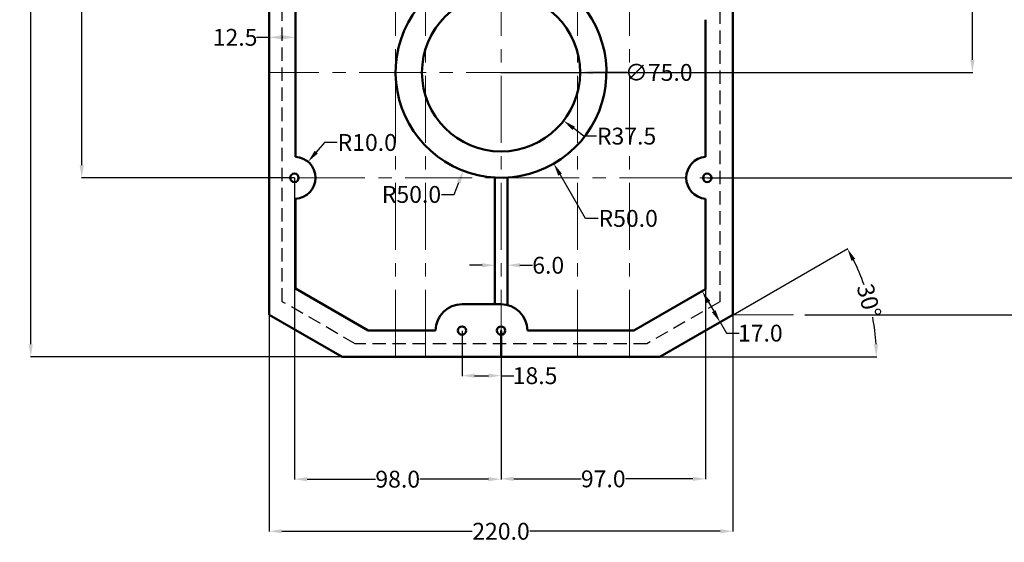
# Model space of a CAD drawing. Units: inches. Extents: x 11765 to 12471, y 10149 to 10793.
# Tile 1 of 8: x 11765 to 12232, y 10149 to 10397. Entities that reach past the tile are written whole.
import ezdxf

# ---------------------------------------------------------------- set-up
doc = ezdxf.new("R2010")
doc.units = ezdxf.units.IN
doc.header["$MEASUREMENT"] = 0
doc.linetypes.add('CENTER', pattern=[50.8, 31.75, -6.35, 6.35, -6.35])
doc.linetypes.add('HIDDEN', pattern=[9.525, 6.35, -3.175])
for name, color, linetype, lineweight in [('M-CNTR', 30, 'CENTER', 18), ('M-DIMS', 2, 'Continuous', 25), ('M-HIDN', 41, 'HIDDEN', 25), ('M-OUTL', 7, 'Continuous', 50)]:
    doc.layers.add(name, color=color, linetype=linetype, lineweight=lineweight)
doc.styles.get("Standard").update_dxf_attribs({"font": 'arial.ttf'})
doc.dimstyles.get("Standard").update_dxf_attribs({"dimtxt": 8, "dimasz": 6, "dimexe": 0.18, "dimexo": 0.0625, "dimgap": 0.09, "dimtad": 0, "dimtoh": 1, "dimdec": 1, "dimzin": 0, "dimdsep": 46, "dimtxsty": 'Standard', "dimcen": 0.09, "dimadec": 0, "dimazin": 0, "dimtfac": 1, "dimtdec": 1, "dimtofl": 0, "dimtmove": 0, "dimatfit": 3, "dimfxl": 1, "dimtolj": 1, "dimtzin": 0, "dimarcsym": 0})

# ---------------------------------------------------------------- blocks, each defined once
blk = doc.blocks.new('*D6')
at = {"layer": 'Defpoints', "color": 0, "transparency": 16777216}
for p in [(11882.91, 10712.15), (11769.87, 10237.15), (11917.55, 10237.15)]:
    blk.add_point(p, dxfattribs=at)
at = {"layer": 'M-DIMS', "color": 0, "lineweight": -2, "transparency": 16777216}
for p, q in [((11882.85, 10712.15), (11769.69, 10712.15)), ((11769.87, 10706.15), (11769.87, 10488.38)), ((11769.87, 10243.15), (11769.87, 10460.91)), ((11917.49, 10237.15), (11769.69, 10237.15))]:
    blk.add_line(p, q, dxfattribs=at)
at = {"layer": 'M-DIMS', "color": 0, "transparency": 16777216}
for points in [[(11768.87, 10706.15), (11770.87, 10706.15), (11769.87, 10712.15)], [(11768.87, 10243.15), (11770.87, 10243.15), (11769.87, 10237.15)]]:
    blk.add_solid(points, dxfattribs=at)
at = {"layer": 'M-DIMS', "color": 0, "transparency": 16777216, "insert": (11769.87, 10474.65), "char_height": 8, "attachment_point": 5, "rotation": 90}
blk.add_mtext('\\A1;475.0', dxfattribs=at)
blk = doc.blocks.new('*D14')
at = {"layer": 'Defpoints', "color": 0, "transparency": 16777216}
for p in [(12156.23, 10592.15), (12216.5, 10592.15), (11992.91, 10372.15)]:
    blk.add_point(p, dxfattribs=at)
at = {"layer": 'M-DIMS', "color": 0, "lineweight": -2, "transparency": 16777216}
for p, q in [((12156.3, 10592.15), (12216.68, 10592.15)), ((12216.5, 10586.15), (12216.5, 10495.79)), ((12216.5, 10378.15), (12216.5, 10468.5)), ((11992.97, 10372.15), (12216.68, 10372.15))]:
    blk.add_line(p, q, dxfattribs=at)
at = {"layer": 'M-DIMS', "color": 0, "transparency": 16777216}
for points in [[(12215.5, 10586.15), (12217.5, 10586.15), (12216.5, 10592.15)], [(12215.5, 10378.15), (12217.5, 10378.15), (12216.5, 10372.15)]]:
    blk.add_solid(points, dxfattribs=at)
at = {"layer": 'M-DIMS', "color": 0, "transparency": 16777216, "insert": (12216.5, 10482.15), "char_height": 8, "attachment_point": 5, "rotation": 90}
blk.add_mtext('\\A1;220.0', dxfattribs=at)
blk = doc.blocks.new('*D15')
at = {"layer": 'Defpoints', "color": 0, "transparency": 16777216}
for p in [(12198.7, 10592.15), (12090.75, 10322.15), (12241.87, 10322.15)]:
    blk.add_point(p, dxfattribs=at)
at = {"layer": 'M-DIMS', "color": 0, "lineweight": -2, "transparency": 16777216}
for p, q in [((12198.76, 10592.15), (12242.05, 10592.15)), ((12241.87, 10586.15), (12241.87, 10470.79)), ((12241.87, 10328.15), (12241.87, 10443.5)), ((12090.81, 10322.15), (12242.05, 10322.15))]:
    blk.add_line(p, q, dxfattribs=at)
at = {"layer": 'M-DIMS', "color": 0, "transparency": 16777216}
for points in [[(12240.87, 10586.15), (12242.87, 10586.15), (12241.87, 10592.15)], [(12240.87, 10328.15), (12242.87, 10328.15), (12241.87, 10322.15)]]:
    blk.add_solid(points, dxfattribs=at)
at = {"layer": 'M-DIMS', "color": 0, "transparency": 16777216, "insert": (12241.87, 10457.15), "char_height": 8, "attachment_point": 5, "rotation": 90}
blk.add_mtext('\\A1;270.0', dxfattribs=at)
blk = doc.blocks.new('*D16')
at = {"layer": 'Defpoints', "color": 0, "transparency": 16777216}
for p in [(12136.92, 10322.15), (12136.92, 10257.15), (12239.74, 10257.15)]:
    blk.add_point(p, dxfattribs=at)
at = {"layer": 'M-DIMS', "color": 0, "lineweight": -2, "transparency": 16777216}
for p, q in [((12136.98, 10322.15), (12239.92, 10322.15)), ((12239.74, 10316.15), (12239.74, 10300.13)), ((12239.74, 10263.15), (12239.74, 10279.16)), ((12136.98, 10257.15), (12239.92, 10257.15))]:
    blk.add_line(p, q, dxfattribs=at)
at = {"layer": 'M-DIMS', "color": 0, "transparency": 16777216}
for points in [[(12238.74, 10316.15), (12240.74, 10316.15), (12239.74, 10322.15)], [(12238.74, 10263.15), (12240.74, 10263.15), (12239.74, 10257.15)]]:
    blk.add_solid(points, dxfattribs=at)
at = {"layer": 'M-DIMS', "color": 0, "transparency": 16777216, "insert": (12239.74, 10289.65), "char_height": 8, "attachment_point": 5, "rotation": 90}
blk.add_mtext('\\A1;65.0', dxfattribs=at)
blk = doc.blocks.new('*D17')
at = {"layer": 'Defpoints', "color": 0, "transparency": 16777216}
for p in [(12102.91, 10257.15), (12169.38, 10254.97), (11917.55, 10237.15), (12068.27, 10237.15), (12068.27, 10237.15)]:
    blk.add_point(p, dxfattribs=at)
at = {"layer": 'M-DIMS', "color": 0, "lineweight": -2, "transparency": 16777216}
for p, q in [((12102.97, 10257.18), (12157.34, 10288.57)), ((12068.33, 10237.15), (12171.12, 10237.15))]:
    blk.add_line(p, q, dxfattribs=at)
for start, end in [(19.4324, 26.6511), (3.3489, 10.5676)]:
    blk.add_arc((12068.27, 10237.15), 102.67, start, end, dxfattribs=at)
at = {"layer": 'M-DIMS', "color": 0, "transparency": 16777216}
for points in [[(12159.15, 10282.72), (12160.91, 10283.67), (12157.18, 10288.48)], [(12171.76, 10243.17), (12169.76, 10243.11), (12170.94, 10237.15)]]:
    blk.add_solid(points, dxfattribs=at)
at = {"layer": 'M-DIMS', "color": 0, "transparency": 16777216, "insert": (12167.44, 10263.72), "char_height": 8, "attachment_point": 5, "rotation": 285}
blk.add_mtext('\\A1;30°', dxfattribs=at)
blk = doc.blocks.new('*D18')
at = {"layer": 'Defpoints', "color": 0, "transparency": 16777216}
for p in [(11882.91, 10257.15), (12102.91, 10257.15), (12102.91, 10154.4)]:
    blk.add_point(p, dxfattribs=at)
at = {"layer": 'M-DIMS', "color": 0, "lineweight": -2, "transparency": 16777216}
for p, q in [((11882.91, 10257.08), (11882.91, 10154.22)), ((12102.91, 10257.08), (12102.91, 10154.22)), ((11888.91, 10154.4), (11979.27, 10154.4)), ((12096.91, 10154.4), (12006.55, 10154.4))]:
    blk.add_line(p, q, dxfattribs=at)
at = {"layer": 'M-DIMS', "color": 0, "transparency": 16777216}
for points in [[(11888.91, 10155.4), (11888.91, 10153.4), (11882.91, 10154.4)], [(12096.91, 10155.4), (12096.91, 10153.4), (12102.91, 10154.4)]]:
    blk.add_solid(points, dxfattribs=at)
at = {"layer": 'M-DIMS', "color": 0, "transparency": 16777216, "insert": (11992.91, 10154.4), "char_height": 8, "attachment_point": 5}
blk.add_mtext('\\A1;220.0', dxfattribs=at)
blk = doc.blocks.new('*D19')
at = {"layer": 'Defpoints', "color": 0, "transparency": 16777216}
for p in [(12074.77, 10260.53), (12096.81, 10253.62), (12083.27, 10245.8)]:
    blk.add_point(p, dxfattribs=at)
at = {"layer": 'M-DIMS', "color": 0, "lineweight": -2, "transparency": 16777216}
for p, q in [((12074.82, 10260.56), (12088.46, 10268.43)), ((12091.31, 10263.15), (12093.81, 10258.82)), ((12083.32, 10245.83), (12096.96, 10253.71)), ((12096.81, 10253.62), (12099.81, 10248.42)), ((12099.81, 10248.42), (12105.81, 10248.42))]:
    blk.add_line(p, q, dxfattribs=at)
at = {"layer": 'M-DIMS', "color": 0, "transparency": 16777216}
for points in [[(12092.17, 10263.65), (12090.44, 10262.65), (12088.31, 10268.34)], [(12094.67, 10259.32), (12092.94, 10258.32), (12096.81, 10253.62)]]:
    blk.add_solid(points, dxfattribs=at)
at = {"layer": 'M-DIMS', "color": 0, "transparency": 16777216, "insert": (12115.9, 10248.42), "char_height": 8, "attachment_point": 5}
blk.add_mtext('\\A1;17.0', dxfattribs=at)
blk = doc.blocks.new('*D20')
at = {"layer": 'Defpoints', "color": 0, "transparency": 16777216}
for p in [(11894.91, 10322.15), (11992.91, 10249.65), (11992.91, 10179.12)]:
    blk.add_point(p, dxfattribs=at)
at = {"layer": 'M-DIMS', "color": 0, "lineweight": -2, "transparency": 16777216}
for p, q in [((11894.91, 10322.08), (11894.91, 10178.94)), ((11992.91, 10249.58), (11992.91, 10178.94)), ((11900.91, 10179.12), (11933.45, 10179.12)), ((11986.91, 10179.12), (11954.38, 10179.12))]:
    blk.add_line(p, q, dxfattribs=at)
at = {"layer": 'M-DIMS', "color": 0, "transparency": 16777216}
for points in [[(11900.91, 10180.12), (11900.91, 10178.12), (11894.91, 10179.12)], [(11986.91, 10180.12), (11986.91, 10178.12), (11992.91, 10179.12)]]:
    blk.add_solid(points, dxfattribs=at)
at = {"layer": 'M-DIMS', "color": 0, "transparency": 16777216, "insert": (11943.91, 10179.12), "char_height": 8, "attachment_point": 5}
blk.add_mtext('\\A1;98.0', dxfattribs=at)
blk = doc.blocks.new('*D21')
at = {"layer": 'Defpoints', "color": 0, "transparency": 16777216}
for p in [(12089.91, 10269.27), (11992.91, 10249.65), (11992.91, 10179.27)]:
    blk.add_point(p, dxfattribs=at)
at = {"layer": 'M-DIMS', "color": 0, "lineweight": -2, "transparency": 16777216}
for p, q in [((12089.91, 10269.21), (12089.91, 10179.09)), ((11992.91, 10249.58), (11992.91, 10179.09)), ((11998.91, 10179.27), (12030.95, 10179.27)), ((12083.91, 10179.27), (12051.88, 10179.27))]:
    blk.add_line(p, q, dxfattribs=at)
at = {"layer": 'M-DIMS', "color": 0, "transparency": 16777216}
for points in [[(11998.91, 10180.27), (11998.91, 10178.27), (11992.91, 10179.27)], [(12083.91, 10180.27), (12083.91, 10178.27), (12089.91, 10179.27)]]:
    blk.add_solid(points, dxfattribs=at)
at = {"layer": 'M-DIMS', "color": 0, "transparency": 16777216, "insert": (12041.41, 10179.27), "char_height": 8, "attachment_point": 5}
blk.add_mtext('\\A1;97.0', dxfattribs=at)
blk = doc.blocks.new('*D22')
at = {"layer": 'Defpoints', "color": 0, "transparency": 16777216}
for p in [(11995.91, 10280.64), (11989.91, 10277.99), (11995.91, 10277.99)]:
    blk.add_point(p, dxfattribs=at)
at = {"layer": 'M-DIMS', "color": 0, "lineweight": -2, "transparency": 16777216}
for p, q in [((11983.91, 10280.64), (11977.91, 10280.64)), ((11989.91, 10278.05), (11989.91, 10280.82)), ((11995.91, 10278.05), (11995.91, 10280.82)), ((12001.91, 10280.64), (12007.91, 10280.64))]:
    blk.add_line(p, q, dxfattribs=at)
at = {"layer": 'M-DIMS', "color": 0, "transparency": 16777216}
for points in [[(11983.91, 10281.64), (11983.91, 10279.64), (11989.91, 10280.64)], [(12001.91, 10281.64), (12001.91, 10279.64), (11995.91, 10280.64)]]:
    blk.add_solid(points, dxfattribs=at)
at = {"layer": 'M-DIMS', "color": 0, "transparency": 16777216, "insert": (12015.29, 10280.64), "char_height": 8, "attachment_point": 5}
blk.add_mtext('\\A1;6.0', dxfattribs=at)
blk = doc.blocks.new('*D23')
at = {"layer": 'Defpoints', "color": 0, "transparency": 16777216}
for p in [(11974.41, 10249.65), (11992.91, 10249.65), (11992.91, 10228.23)]:
    blk.add_point(p, dxfattribs=at)
at = {"layer": 'M-DIMS', "color": 0, "lineweight": -2, "transparency": 16777216}
for p, q in [((11974.41, 10249.58), (11974.41, 10228.05)), ((11992.91, 10249.58), (11992.91, 10228.05)), ((11980.41, 10228.23), (11986.91, 10228.23)), ((11992.91, 10228.23), (11998.91, 10228.23))]:
    blk.add_line(p, q, dxfattribs=at)
at = {"layer": 'M-DIMS', "color": 0, "transparency": 16777216}
for points in [[(11980.41, 10229.23), (11980.41, 10227.23), (11974.41, 10228.23)], [(11986.91, 10229.23), (11986.91, 10227.23), (11992.91, 10228.23)]]:
    blk.add_solid(points, dxfattribs=at)
at = {"layer": 'M-DIMS', "color": 0, "transparency": 16777216, "insert": (12009.05, 10228.23), "char_height": 8, "attachment_point": 5}
blk.add_mtext('\\A1;18.5', dxfattribs=at)
blk = doc.blocks.new('*D29')
at = {"layer": 'Defpoints', "color": 0, "transparency": 16777216}
for p in [(11794.06, 10592.15), (11889.16, 10592.15), (11894.91, 10322.15)]:
    blk.add_point(p, dxfattribs=at)
at = {"layer": 'M-DIMS', "color": 0, "lineweight": -2, "transparency": 16777216}
for p, q in [((11889.1, 10592.15), (11793.88, 10592.15)), ((11794.06, 10586.15), (11794.06, 10470.79)), ((11794.06, 10328.15), (11794.06, 10443.5)), ((11894.85, 10322.15), (11793.88, 10322.15))]:
    blk.add_line(p, q, dxfattribs=at)
at = {"layer": 'M-DIMS', "color": 0, "transparency": 16777216}
for points in [[(11793.06, 10586.15), (11795.06, 10586.15), (11794.06, 10592.15)], [(11793.06, 10328.15), (11795.06, 10328.15), (11794.06, 10322.15)]]:
    blk.add_solid(points, dxfattribs=at)
at = {"layer": 'M-DIMS', "color": 0, "transparency": 16777216, "insert": (11794.06, 10457.15), "char_height": 8, "attachment_point": 5, "rotation": 90}
blk.add_mtext('\\A1;270.0', dxfattribs=at)
blk = doc.blocks.new('*D32')
at = {"layer": 'Defpoints', "color": 0, "transparency": 16777216}
for p in [(11882.91, 10389.52), (11882.91, 10388.8), (11895.41, 10389.52)]:
    blk.add_point(p, dxfattribs=at)
at = {"layer": 'M-DIMS', "color": 0, "lineweight": -2, "transparency": 16777216}
for p, q in [((11882.91, 10388.8), (11876.91, 10388.8)), ((11882.91, 10389.45), (11882.91, 10388.62)), ((11889.41, 10388.8), (11888.91, 10388.8)), ((11895.41, 10389.45), (11895.41, 10388.62))]:
    blk.add_line(p, q, dxfattribs=at)
at = {"layer": 'M-DIMS', "color": 0, "transparency": 16777216}
for points in [[(11888.91, 10389.8), (11888.91, 10387.8), (11882.91, 10388.8)], [(11889.41, 10389.8), (11889.41, 10387.8), (11895.41, 10388.8)]]:
    blk.add_solid(points, dxfattribs=at)
at = {"layer": 'M-DIMS', "color": 0, "transparency": 16777216, "insert": (11866.78, 10388.8), "char_height": 8, "attachment_point": 5}
blk.add_mtext('\\A1;12.5', dxfattribs=at)
blk = doc.blocks.new('*D44')
at = {"layer": 'Defpoints', "color": 0, "transparency": 16777216}
for p in [(11992.91, 10372.15), (11975.02, 10325.45)]:
    blk.add_point(p, dxfattribs=at)
at = {"layer": 'M-DIMS', "color": 0, "lineweight": -2, "transparency": 16777216}
for p, q in [((11992.82, 10372.15), (11993, 10372.15)), ((11992.91, 10372.06), (11992.91, 10372.24)), ((11970.73, 10314.25), (11972.88, 10319.85)), ((11964.73, 10314.25), (11970.73, 10314.25))]:
    blk.add_line(p, q, dxfattribs=at)
at = {"layer": 'M-DIMS', "color": 0, "transparency": 16777216}
blk.add_solid([(11971.94, 10320.21), (11973.81, 10319.49), (11975.02, 10325.45)], dxfattribs=at)
at = {"layer": 'M-DIMS', "color": 0, "transparency": 16777216, "insert": (11950.44, 10314.25), "char_height": 8, "attachment_point": 5}
blk.add_mtext('\\A1;R50.0', dxfattribs=at)
blk = doc.blocks.new('*D45')
at = {"layer": 'Defpoints', "color": 0, "transparency": 16777216}
for p in [(11992.91, 10372.15), (12022.61, 10349.25)]:
    blk.add_point(p, dxfattribs=at)
at = {"layer": 'M-DIMS', "color": 0, "lineweight": -2, "transparency": 16777216}
for p, q in [((11992.82, 10372.15), (11993, 10372.15)), ((11992.91, 10372.06), (11992.91, 10372.24)), ((12032.12, 10341.93), (12027.37, 10345.59)), ((12038.12, 10341.93), (12032.12, 10341.93))]:
    blk.add_line(p, q, dxfattribs=at)
at = {"layer": 'M-DIMS', "color": 0, "transparency": 16777216}
blk.add_solid([(12027.98, 10346.38), (12026.76, 10344.8), (12022.61, 10349.25)], dxfattribs=at)
at = {"layer": 'M-DIMS', "color": 0, "transparency": 16777216, "insert": (12052.46, 10341.93), "char_height": 8, "attachment_point": 5}
blk.add_mtext('\\A1;R37.5', dxfattribs=at)
blk = doc.blocks.new('*D50')
at = {"layer": 'Defpoints', "color": 0, "transparency": 16777216}
for p in [(11901.39, 10329.76), (11894.91, 10322.15)]:
    blk.add_point(p, dxfattribs=at)
at = {"layer": 'M-DIMS', "color": 0, "lineweight": -2, "transparency": 16777216}
for p, q in [((11909.17, 10338.9), (11905.28, 10334.33)), ((11915.17, 10338.9), (11909.17, 10338.9)), ((11894.82, 10322.15), (11895, 10322.15)), ((11894.91, 10322.06), (11894.91, 10322.24))]:
    blk.add_line(p, q, dxfattribs=at)
at = {"layer": 'M-DIMS', "color": 0, "transparency": 16777216}
blk.add_solid([(11904.52, 10334.98), (11906.04, 10333.68), (11901.39, 10329.76)], dxfattribs=at)
at = {"layer": 'M-DIMS', "color": 0, "transparency": 16777216, "insert": (11929.47, 10338.9), "char_height": 8, "attachment_point": 5}
blk.add_mtext('\\A1;R10.0', dxfattribs=at)
blk = doc.blocks.new('*D67')
at = {"layer": 'Defpoints', "color": 0, "transparency": 16777216}
for p in [(11992.91, 10372.15), (12017.93, 10328.85)]:
    blk.add_point(p, dxfattribs=at)
at = {"layer": 'M-DIMS', "color": 0, "lineweight": -2, "transparency": 16777216}
for p, q in [((11992.82, 10372.15), (11993, 10372.15)), ((11992.91, 10372.06), (11992.91, 10372.24)), ((12032.94, 10302.88), (12020.93, 10323.66)), ((12038.94, 10302.88), (12032.94, 10302.88))]:
    blk.add_line(p, q, dxfattribs=at)
at = {"layer": 'M-DIMS', "color": 0, "transparency": 16777216}
blk.add_solid([(12021.79, 10324.16), (12020.06, 10323.16), (12017.93, 10328.85)], dxfattribs=at)
at = {"layer": 'M-DIMS', "color": 0, "transparency": 16777216, "insert": (12053.23, 10302.88), "char_height": 8, "attachment_point": 5}
blk.add_mtext('\\A1;R50.0', dxfattribs=at)
blk = doc.blocks.new('*D70')
at = {"layer": 'Defpoints', "color": 0, "transparency": 16777216}
for p in [(11955.41, 10372.15), (12030.41, 10372.15)]:
    blk.add_point(p, dxfattribs=at)
at = {"layer": 'M-DIMS', "color": 0, "lineweight": -2, "transparency": 16777216}
for p, q in [((11992.82, 10372.15), (11993, 10372.15)), ((11992.91, 10372.06), (11992.91, 10372.24)), ((12052.91, 10372.15), (12036.41, 10372.15))]:
    blk.add_line(p, q, dxfattribs=at)
at = {"layer": 'M-DIMS', "color": 0, "transparency": 16777216}
blk.add_solid([(12036.41, 10373.15), (12036.41, 10371.15), (12030.41, 10372.15)], dxfattribs=at)
at = {"layer": 'M-DIMS', "color": 0, "transparency": 16777216, "insert": (12067.73, 10372.15), "char_height": 8, "attachment_point": 5}
blk.add_mtext('\\A1;∅75.0', dxfattribs=at)

msp = doc.modelspace()

# ---------------------------------------------------------------- linework, layer by layer
at = {"layer": 'M-CNTR'}
for p, q in [((11942.912, 10237.146), (11942.912, 10712.146)), ((11957.122, 10237.146), (11957.122, 10712.146)), ((11992.912, 10237.146), (11992.912, 10712.146)), ((12029.232, 10237.146), (12029.232, 10712.146)), ((12053.912, 10237.146), (12053.912, 10712.146)), ((12211.379, 10372.146), (11882.912, 10372.146)), ((12182.382, 10322.146), (11882.912, 10322.146)), ((12182.382, 10257.146), (12102.912, 10257.146))]:
    msp.add_line(p, q, dxfattribs=at)
at = {"layer": 'M-HIDN'}
msp.add_lwpolyline([(12060.662, 10705.896), (12060.662, 10515.896), (12096.662, 10515.896), (12096.662, 10263.352), (12062.096, 10243.396), (11923.728, 10243.396), (11889.162, 10263.352), (11889.162, 10705.896)], close=True, dxfattribs=at)
at = {"layer": 'M-OUTL'}
for p, q in [((11882.912, 10712.146), (11882.912, 10257.146)), ((12102.912, 10257.146), (12102.912, 10522.146)), ((11895.412, 10437.158), (11895.412, 10332.133)), ((12089.912, 10332.111), (12089.912, 10397.181)), ((11989.912, 10322.146), (11989.912, 10262.146)), ((11995.912, 10322.146), (11995.912, 10262.146)), ((11895.412, 10312.158), (11895.412, 10269.559)), ((12089.912, 10269.27), (12089.912, 10312.181)), ((11895.412, 10269.559), (11929.902, 10249.646)), ((12089.912, 10269.27), (12055.922, 10249.646)), ((11992.912, 10262.146), (11974.412, 10262.146)), ((11882.912, 10257.146), (11917.553, 10237.146)), ((12102.912, 10257.146), (12068.271, 10237.146)), ((11961.912, 10249.646), (11929.902, 10249.646)), ((11992.912, 10249.646), (11992.912, 10237.146)), ((12055.922, 10249.646), (12005.412, 10249.646)), ((11917.553, 10237.146), (12068.271, 10237.146))]:
    msp.add_line(p, q, dxfattribs=at)
for centre, radius in [((11992.912, 10372.146), 37.5), ((11894.912, 10322.146), 2), ((12090.748, 10322.146), 2), ((11974.412, 10249.646), 2), ((11992.912, 10249.646), 2)]:
    msp.add_circle(centre, radius, dxfattribs=at)
for centre, radius, start, end in [((11992.912, 10372.146), 50, 90, 35.46169), ((11894.912, 10322.146), 10, 272.86598, 87.13402), ((12090.748, 10322.146), 10, 94.79487, 265.20513), ((11974.412, 10249.646), 12.5, 90, 180), ((11992.912, 10249.646), 12.5, 0, 90)]:
    msp.add_arc(centre, radius, start, end, dxfattribs=at)

# ---------------------------------------------------------------- dimensions: what is measured, and where the dimension line sits
at = {"layer": 'M-DIMS'}
for base, p1, p2, picture, middle in [((11769.869, 10237.146), (11882.912, 10712.146), (11917.553, 10237.146), '*D6', (11769.869, 10474.646)), ((11794.063, 10592.146), (11894.912, 10322.146), (11889.162, 10592.146), '*D29', (11794.063, 10457.146)), ((12216.505, 10592.146), (11992.912, 10372.146), (12156.234, 10592.146), '*D14', (12216.505, 10482.146)), ((12241.874, 10322.146), (12198.696, 10592.146), (12090.748, 10322.146), '*D15', (12241.874, 10457.146)), ((12239.736, 10257.146), (12136.919, 10322.146), (12136.919, 10257.146), '*D16', (12239.736, 10289.646))]:
    dim = msp.add_linear_dim(base=base, p1=p1, p2=p2, angle=90, dimstyle='Standard', override={"dimclrd": 0, "dimclre": 0, "dimclrt": 0}, dxfattribs=at)
    dim.commit()
    dim.dimension.update_dxf_attribs({"geometry": picture, "text_midpoint": middle})
for base, p1, p2, picture, middle in [((11882.912, 10388.804), (11895.412, 10389.516), (11882.912, 10389.516), '*D32', (11866.778, 10388.804)), ((11992.912, 10179.124), (11894.912, 10322.146), (11992.912, 10249.646), '*D20', (11943.912, 10179.124)), ((11995.912, 10280.645), (11989.912, 10277.991), (11995.912, 10277.991), '*D22', (12015.293, 10280.645)), ((11992.912, 10179.274), (12089.912, 10269.27), (11992.912, 10249.646), '*D21', (12041.412, 10179.274)), ((12102.912, 10154.397), (11882.912, 10257.146), (12102.912, 10257.146), '*D18', (11992.912, 10154.397)), ((11992.912, 10228.231), (11974.412, 10249.646), (11992.912, 10249.646), '*D23', (12009.046, 10228.231))]:
    dim = msp.add_linear_dim(base=base, p1=p1, p2=p2, dimstyle='Standard', override={"dimclrd": 0, "dimclre": 0, "dimclrt": 0}, dxfattribs=at)
    dim.commit()
    dim.dimension.update_dxf_attribs({"geometry": picture, "text_midpoint": middle})
dim = msp.add_diameter_dim_2p(p1=(11955.412, 10372.145), p2=(12030.412, 10372.146), dimstyle='Standard', override={"dimdec": 1, "dimlfac": 1, "dimrnd": 0, "dimzin": 0, "dimdsep": 46, "dimlunit": 2}, dxfattribs=at)
dim.commit()
dim.dimension.update_dxf_attribs({"geometry": '*D70', "text_midpoint": (12052.912, 10372.146), "dimtype": 163})
for center, mpoint, picture, middle in [((11992.912, 10372.146), (11975.024, 10325.455), '*D44', (11950.436, 10314.249)), ((11992.912, 10372.146), (12022.615, 10349.254), '*D45', (12052.458, 10341.929)), ((11894.912, 10322.146), (11901.393, 10329.761), '*D50', (11929.466, 10338.899))]:
    dim = msp.add_radius_dim(center=center, mpoint=mpoint, dimstyle='Standard', override={"dimclrd": 0, "dimclre": 0, "dimclrt": 0}, dxfattribs=at)
    dim.commit()
    dim.dimension.update_dxf_attribs({"geometry": picture, "text_midpoint": middle})
dim = msp.add_radius_dim(center=(11992.912, 10372.146), mpoint=(12017.927, 10328.853), dimstyle='Standard', override={"dimdec": 1, "dimlfac": 1, "dimrnd": 0, "dimzin": 0, "dimdsep": 46, "dimlunit": 2}, dxfattribs=at)
dim.commit()
dim.dimension.update_dxf_attribs({"geometry": '*D67', "text_midpoint": (12053.231, 10302.878), "dimtype": 164})
dim = msp.add_angular_dim_2l(base=(12169.378, 10254.973), line1=((12102.912, 10257.146), (12068.271, 10237.146)), line2=((11917.553, 10237.146), (12068.271, 10237.146)), dimstyle='Standard', override={"dimclrd": 0, "dimclre": 0, "dimclrt": 0}, dxfattribs=at)
dim.commit()
dim.dimension.update_dxf_attribs({"geometry": '*D17', "text_midpoint": (12167.44, 10263.718)})
dim = msp.add_aligned_dim(p1=(12074.766, 10260.525), p2=(12083.266, 10245.803), distance=15.635, dimstyle='Standard', override={"dimclrd": 0, "dimclre": 0, "dimclrt": 0}, dxfattribs=at)
dim.commit()
dim.dimension.update_dxf_attribs({"geometry": '*D19', "text_midpoint": (12115.896, 10248.424)})

doc.saveas('drawing.dxf')
